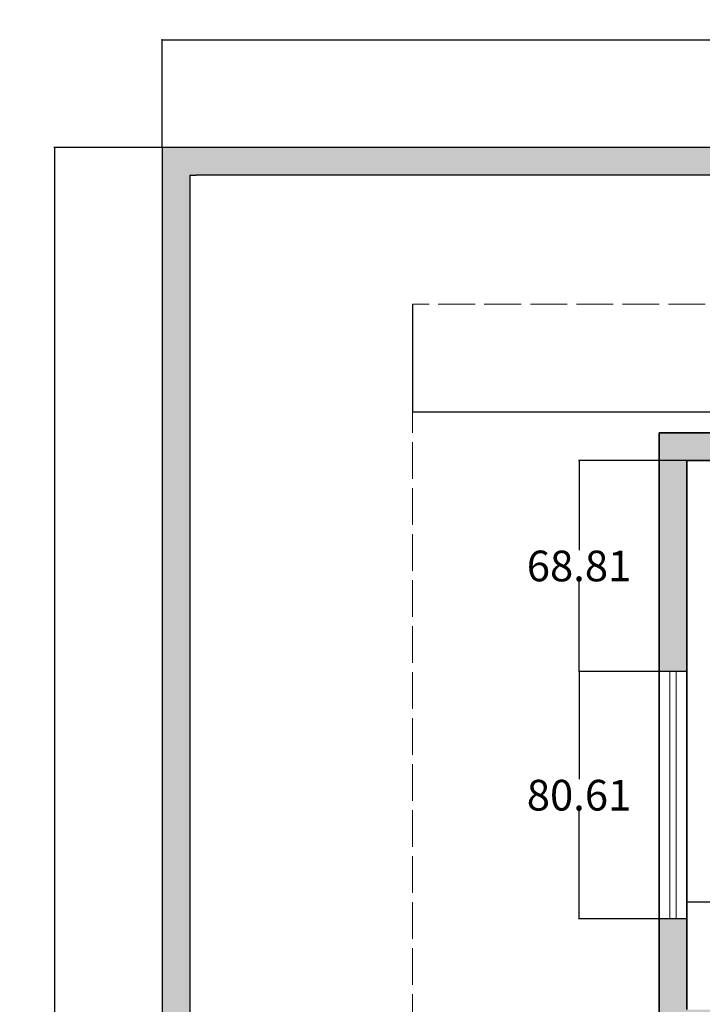
# Model space of a CAD drawing. Units: inches. Extents: x 409 to 1056, y 160 to 945.
# Tile 4 of 6: x 409 to 632, y 624 to 945. Entities that reach past the tile are written whole.
import ezdxf

# ---------------------------------------------------------------- set-up
doc = ezdxf.new("R2010")
doc.units = ezdxf.units.IN
doc.header["$MEASUREMENT"] = 0
doc.linetypes.add('ACAD_ISO02W100', pattern=[15, 12, -3])
for name, color, linetype, lineweight in [('A-ANNO-DIMS', 2, 'Continuous', 18), ('A-GLAZ', 4, 'Continuous', 18), ('A-ROOF-BYND', 8, 'ACAD_ISO02W100', 13), ('A-WALL', 7, 'Continuous', 35), ('A-WALL-PRPT', 7, 'Continuous', 30)]:
    doc.layers.add(name, color=color, linetype=linetype, lineweight=lineweight)
doc.layers.add('A-WALL-PATT', color=251, linetype='Continuous', lineweight=13, true_color=0x636466)
doc.styles.get("Standard").update_dxf_attribs({"font": 'arial.ttf'})
doc.dimstyles.get("Standard").update_dxf_attribs({"dimtxt": 10, "dimasz": 0.18, "dimexe": 0.18, "dimexo": 0.0625, "dimgap": 0.09, "dimtad": 0, "dimtih": 1, "dimtoh": 1, "dimdec": 0, "dimzin": 0, "dimdsep": 46, "dimlunit": 3, "dimtxsty": 'Standard', "dimcen": 0.09, "dimadec": 0, "dimazin": 0, "dimtfac": 1, "dimtdec": 0, "dimtofl": 0, "dimtmove": 0, "dimatfit": 3, "dimfxl": 1, "dimtolj": 1, "dimtzin": 0, "dimarcsym": 0})

# ---------------------------------------------------------------- blocks, each defined once
blk = doc.blocks.new('*D35')
at = {"layer": 'A-ANNO-DIMS', "color": 0, "lineweight": -2, "transparency": 16777216}
for p, q in [((455.74, 903.81), (455.74, 939.05)), ((455.92, 938.87), (702.61, 938.87)), ((971.56, 938.87), (724.88, 938.87)), ((971.74, 903.81), (971.74, 939.05))]:
    blk.add_line(p, q, dxfattribs=at)
at = {"layer": 'A-ANNO-DIMS', "color": 0, "transparency": 16777216}
for points in [[(455.92, 938.9), (455.92, 938.84), (455.74, 938.87)], [(971.56, 938.9), (971.56, 938.84), (971.74, 938.87)]]:
    blk.add_solid(points, dxfattribs=at)
at = {"layer": 'Defpoints', "color": 0, "transparency": 16777216}
for p in [(971.74, 938.87), (455.74, 903.74), (971.74, 903.74)]:
    blk.add_point(p, dxfattribs=at)
at = {"layer": 'A-ANNO-DIMS', "color": 0, "transparency": 16777216, "insert": (713.74, 938.87), "char_height": 10, "attachment_point": 5}
blk.add_mtext('\\A1;516', dxfattribs=at)
blk = doc.blocks.new('*D36')
at = {"layer": 'A-ANNO-DIMS', "color": 0, "lineweight": -2, "transparency": 16777216}
for p, q in [((455.68, 903.74), (420.44, 903.74)), ((420.62, 903.56), (420.62, 557.94)), ((420.62, 201.92), (420.62, 547.55)), ((455.68, 201.74), (420.44, 201.74))]:
    blk.add_line(p, q, dxfattribs=at)
at = {"layer": 'A-ANNO-DIMS', "color": 0, "transparency": 16777216}
for points in [[(420.59, 903.56), (420.65, 903.56), (420.62, 903.74)], [(420.59, 201.92), (420.65, 201.92), (420.62, 201.74)]]:
    blk.add_solid(points, dxfattribs=at)
at = {"layer": 'Defpoints', "color": 0, "transparency": 16777216}
for p in [(420.62, 903.74), (455.74, 903.74), (455.74, 201.74)]:
    blk.add_point(p, dxfattribs=at)
at = {"layer": 'A-ANNO-DIMS', "color": 0, "transparency": 16777216, "insert": (420.62, 552.74), "char_height": 10, "attachment_point": 5}
blk.add_mtext('\\A1;702', dxfattribs=at)
blk = doc.blocks.new('*D46')
at = {"layer": 'A-ANNO-DIMS', "color": 0, "lineweight": -2, "transparency": 16777216}
for p, q in [((626.68, 732.93), (591.44, 732.93)), ((591.62, 732.75), (591.62, 697.82)), ((591.62, 652.5), (591.62, 687.43)), ((626.68, 652.32), (591.44, 652.32))]:
    blk.add_line(p, q, dxfattribs=at)
at = {"layer": 'A-ANNO-DIMS', "color": 0, "transparency": 16777216}
for points in [[(591.59, 732.75), (591.65, 732.75), (591.62, 732.93)], [(591.59, 652.5), (591.65, 652.5), (591.62, 652.32)]]:
    blk.add_solid(points, dxfattribs=at)
at = {"layer": 'Defpoints', "color": 0, "transparency": 16777216}
for p in [(591.62, 732.93), (626.74, 732.93), (626.74, 652.32)]:
    blk.add_point(p, dxfattribs=at)
at = {"layer": 'A-ANNO-DIMS', "color": 0, "transparency": 16777216, "insert": (591.62, 692.62), "char_height": 10, "attachment_point": 5}
blk.add_mtext('\\A1;80.61', dxfattribs=at)
blk = doc.blocks.new('*D47')
at = {"layer": 'A-ANNO-DIMS', "color": 0, "lineweight": -2, "transparency": 16777216}
for p, q in [((626.68, 801.74), (591.44, 801.74)), ((591.62, 801.56), (591.62, 772.53)), ((591.62, 733.11), (591.62, 762.14)), ((626.68, 732.93), (591.44, 732.93))]:
    blk.add_line(p, q, dxfattribs=at)
at = {"layer": 'A-ANNO-DIMS', "color": 0, "transparency": 16777216}
for points in [[(591.59, 801.56), (591.65, 801.56), (591.62, 801.74)], [(591.59, 733.11), (591.65, 733.11), (591.62, 732.93)]]:
    blk.add_solid(points, dxfattribs=at)
at = {"layer": 'Defpoints', "color": 0, "transparency": 16777216}
for p in [(591.62, 801.74), (626.74, 801.74), (626.74, 732.93)]:
    blk.add_point(p, dxfattribs=at)
at = {"layer": 'A-ANNO-DIMS', "color": 0, "transparency": 16777216, "insert": (591.62, 767.34), "char_height": 10, "attachment_point": 5}
blk.add_mtext('\\A1;68.81', dxfattribs=at)
blk = doc.blocks.new('*D54')
at = {"layer": 'A-ANNO-DIMS', "color": 0, "lineweight": -2, "transparency": 16777216}
for p, q in [((626.74, 622.81), (626.74, 658.05)), ((649.64, 622.81), (649.64, 658.05)), ((626.92, 657.87), (649.46, 657.87)), ((649.64, 657.87), (649.82, 657.87))]:
    blk.add_line(p, q, dxfattribs=at)
at = {"layer": 'A-ANNO-DIMS', "color": 0, "transparency": 16777216}
for points in [[(626.92, 657.9), (626.92, 657.84), (626.74, 657.87)], [(649.46, 657.9), (649.46, 657.84), (649.64, 657.87)]]:
    blk.add_solid(points, dxfattribs=at)
at = {"layer": 'Defpoints', "color": 0, "transparency": 16777216}
for p in [(649.64, 657.87), (626.74, 622.74), (649.64, 622.74)]:
    blk.add_point(p, dxfattribs=at)
at = {"layer": 'A-ANNO-DIMS', "color": 0, "transparency": 16777216, "insert": (663, 657.87), "char_height": 10, "attachment_point": 5}
blk.add_mtext('\\A1;22.9', dxfattribs=at)
blk = doc.blocks.new('*D60')
at = {"layer": 'A-ANNO-DIMS', "color": 0, "lineweight": -2, "transparency": 16777216}
for p, q in [((537.3, 852.68), (537.3, 817.44)), ((962.74, 852.68), (962.74, 817.44)), ((537.48, 817.62), (728.99, 817.62)), ((962.56, 817.62), (771.05, 817.62))]:
    blk.add_line(p, q, dxfattribs=at)
at = {"layer": 'A-ANNO-DIMS', "color": 0, "transparency": 16777216}
for points in [[(537.48, 817.65), (537.48, 817.59), (537.3, 817.62)], [(962.56, 817.65), (962.56, 817.59), (962.74, 817.62)]]:
    blk.add_solid(points, dxfattribs=at)
at = {"layer": 'Defpoints', "color": 0, "transparency": 16777216}
for p in [(537.3, 852.74), (962.74, 852.74), (537.3, 817.62)]:
    blk.add_point(p, dxfattribs=at)
at = {"layer": 'A-ANNO-DIMS', "color": 0, "transparency": 16777216, "insert": (750.02, 817.62), "char_height": 10, "attachment_point": 5}
blk.add_mtext('\\A1;425.44', dxfattribs=at)

msp = doc.modelspace()

# ---------------------------------------------------------------- hatches: boundary and pattern name
at = {"layer": 'A-WALL-PATT'}
h = msp.add_hatch(color=256, dxfattribs=at)
h.dxf.hatch_style = 1
h.paths.add_polyline_path([(730.4481, 698.1956), (696.9841, 709.3369, 1), (696.9841, 678.8752)], flags=17)
h.paths.add_polyline_path([(803.8768, 698.1956), (770.4128, 709.3369, 1), (770.4128, 678.8752)], flags=17)
h.paths.add_polyline_path([(464.7418, 894.7439), (466.7418, 894.7439), (962.7418, 894.7439), (962.7418, 810.7439), (971.7418, 810.7439), (971.7418, 903.7439), (455.7418, 903.7439), (455.7418, 201.7439), (971.7418, 201.7439), (971.7418, 240.7439), (962.7418, 240.7439), (962.7418, 210.7439), (464.7418, 210.7439)])
h = msp.add_hatch(color=256, dxfattribs=at)
h.dxf.hatch_style = 1
h.paths.add_polyline_path([(626.7418, 801.7439), (870.7418, 801.7439), (870.7418, 710.7439), (870.7418, 683.9043), (875.7418, 683.9043), (875.7418, 707.7439), (962.7418, 707.7439), (962.7418, 710.7439), (875.7418, 710.7439), (875.7418, 722.7439), (875.7418, 801.7439), (885.6955, 801.7439, -0.06325422), (884.5523, 810.7439), (617.7418, 810.7439), (617.7418, 732.9297), (626.7418, 732.9297)])
h.paths.add_polyline_path([(962.7418, 810.7439), (920.5523, 810.7439), (920.5523, 801.7439), (962.7418, 801.7439)], flags=17)
h.paths.add_polyline_path([(971.7418, 810.7439), (962.7418, 810.7439), (962.7418, 801.7439), (962.7418, 707.7439), (962.7418, 622.7439), (962.7418, 613.7439), (962.7418, 548.7439), (856.7418, 548.7439), (847.7418, 548.7439), (776.7418, 548.7439), (776.7418, 569.8172), (768.7418, 569.8172), (768.7418, 539.7439), (847.7418, 539.7439), (971.7418, 539.7439), (971.7418, 613.7439), (971.7418, 707.7439)])
h.paths.add_polyline_path([(883.2418, 622.7439), (875.7418, 622.7439), (684.4993, 622.7439, -0.06325422), (685.6424, 613.7439), (870.7418, 613.7439), (875.7418, 613.7439), (884.3849, 613.7439, -0.06325422)])
h.paths.add_polyline_path([(649.6424, 622.7439), (626.7418, 622.7439), (626.7418, 613.7439), (649.6424, 613.7439)])
h.paths.add_polyline_path([(626.7418, 652.3165), (617.7418, 652.3165), (617.7418, 613.7439), (626.7418, 613.7439), (626.7418, 622.7439)])
h.paths.add_polyline_path([(776.7418, 613.7439), (768.7418, 613.7439), (768.7418, 590.4138), (776.7418, 590.4138)], flags=17)
h.paths.add_polyline_path([(856.7418, 613.7439), (847.7418, 613.7439), (847.7418, 548.7439), (856.7418, 548.7439)], flags=17)
h.paths.add_polyline_path([(962.7418, 622.7439), (919.2418, 622.7439), (919.2418, 613.7439), (962.7418, 613.7439)], flags=17)
h.paths.add_polyline_path([(971.7418, 539.7439), (962.7418, 539.7439), (962.7418, 452.7439), (687.1506, 452.7439, -0.06325422), (686.0074, 443.7439), (962.7418, 443.7439), (962.7418, 331.7439), (927.6873, 331.7439, -0.02784244), (927.9102, 327.7439), (962.7418, 327.7439), (962.7418, 249.7439), (871.7418, 249.7439), (870.7418, 249.7439), (626.7418, 249.7439), (626.7418, 282.7439), (617.7418, 282.7439), (617.7418, 240.7439), (870.7418, 240.7439), (871.7418, 240.7439), (971.7418, 240.7439), (971.7418, 249.7439), (971.7418, 327.7439), (971.7418, 331.7439), (971.7418, 443.7439), (971.7418, 452.7439)])
h.paths.add_polyline_path([(875.7418, 443.7439), (870.7418, 443.7439), (870.7418, 327.7439), (871.7418, 327.7439), (891.9102, 327.7439), (891.9102, 331.7439), (875.7418, 331.7439)], flags=17)

# ---------------------------------------------------------------- linework, layer by layer
at = {"layer": 'A-GLAZ'}
for p, q in [((626.7418, 732.9297), (617.7418, 732.9297)), ((621.2418, 732.9297), (621.2418, 652.3165)), ((623.2418, 732.9297), (623.2418, 652.3165)), ((626.7418, 652.3165), (617.7418, 652.3165))]:
    msp.add_line(p, q, dxfattribs=at)
at = {"layer": 'A-ROOF-BYND'}
for p, q in [((962.7418, 852.7439), (537.2978, 852.7439)), ((537.2978, 852.7439), (537.2978, 223.8898))]:
    msp.add_line(p, q, dxfattribs=at)
at = {"layer": 'A-WALL'}
for p, q in [((617.7418, 810.7439), (617.7418, 613.7439)), ((884.5523, 810.7439), (617.7418, 810.7439)), ((870.7418, 801.7439), (626.7418, 801.7439)), ((626.7418, 801.7439), (626.7418, 622.7439))]:
    msp.add_line(p, q, dxfattribs=at)
at = {"layer": 'A-WALL-PRPT'}
for p, q in [((455.7418, 903.7439), (455.7418, 201.7439)), ((971.7418, 903.7439), (455.7418, 903.7439)), ((464.7418, 894.7439), (466.7418, 894.7439)), ((464.7418, 894.7439), (464.7418, 210.7439)), ((962.7418, 894.7439), (466.7418, 894.7439))]:
    msp.add_line(p, q, dxfattribs=at)

# ---------------------------------------------------------------- dimensions: what is measured, and where the dimension line sits
at = {"layer": 'A-ANNO-DIMS'}
for base, p1, p2, override, picture, middle in [((971.7418, 938.8689), (455.7418, 903.7439), (971.7418, 903.7439), {"dimdec": 0, "dimlfac": 1, "dimrnd": 0, "dimzin": 0, "dimdsep": 46, "dimlunit": 2}, '*D35', (713.7418, 938.8689)), ((649.6424, 657.8689), (626.7418, 622.7439), (649.6424, 622.7439), {"dimdec": 1, "dimlfac": 1, "dimrnd": 0, "dimzin": 0, "dimdsep": 46, "dimlunit": 2}, '*D54', (662.9956, 657.8689))]:
    dim = msp.add_linear_dim(base=base, p1=p1, p2=p2, dimstyle='Standard', override=override, dxfattribs=at)
    dim.commit()
    dim.dimension.update_dxf_attribs({"geometry": picture, "text_midpoint": middle})
for base, p1, p2, angle, override, picture, middle in [((420.6168, 903.7439), (455.7418, 201.7439), (455.7418, 903.7439), 90, {"dimdec": 0, "dimlfac": 1, "dimrnd": 0, "dimzin": 0, "dimdsep": 46, "dimlunit": 2}, '*D36', (420.6168, 552.7439)), ((537.2978, 817.6189), (962.7418, 852.7439), (537.2978, 852.7439), 180, {"dimdec": 2, "dimlfac": 1, "dimrnd": 0, "dimzin": 0, "dimdsep": 46, "dimlunit": 2}, '*D60', (750.0198, 817.6189)), ((591.6168, 801.7439), (626.7418, 732.9297), (626.7418, 801.7439), 90, {"dimdec": 2, "dimlfac": 1, "dimrnd": 0, "dimzin": 0, "dimdsep": 46, "dimlunit": 2}, '*D47', (591.6168, 767.3368)), ((591.6168, 732.9297), (626.7418, 652.3165), (626.7418, 732.9297), 90, {"dimdec": 2, "dimlfac": 1, "dimrnd": 0, "dimzin": 0, "dimdsep": 46, "dimlunit": 2}, '*D46', (591.6168, 692.6231))]:
    dim = msp.add_linear_dim(base=base, p1=p1, p2=p2, angle=angle, dimstyle='Standard', override=override, dxfattribs=at)
    dim.commit()
    dim.dimension.update_dxf_attribs({"geometry": picture, "text_midpoint": middle})

doc.saveas('drawing.dxf')
